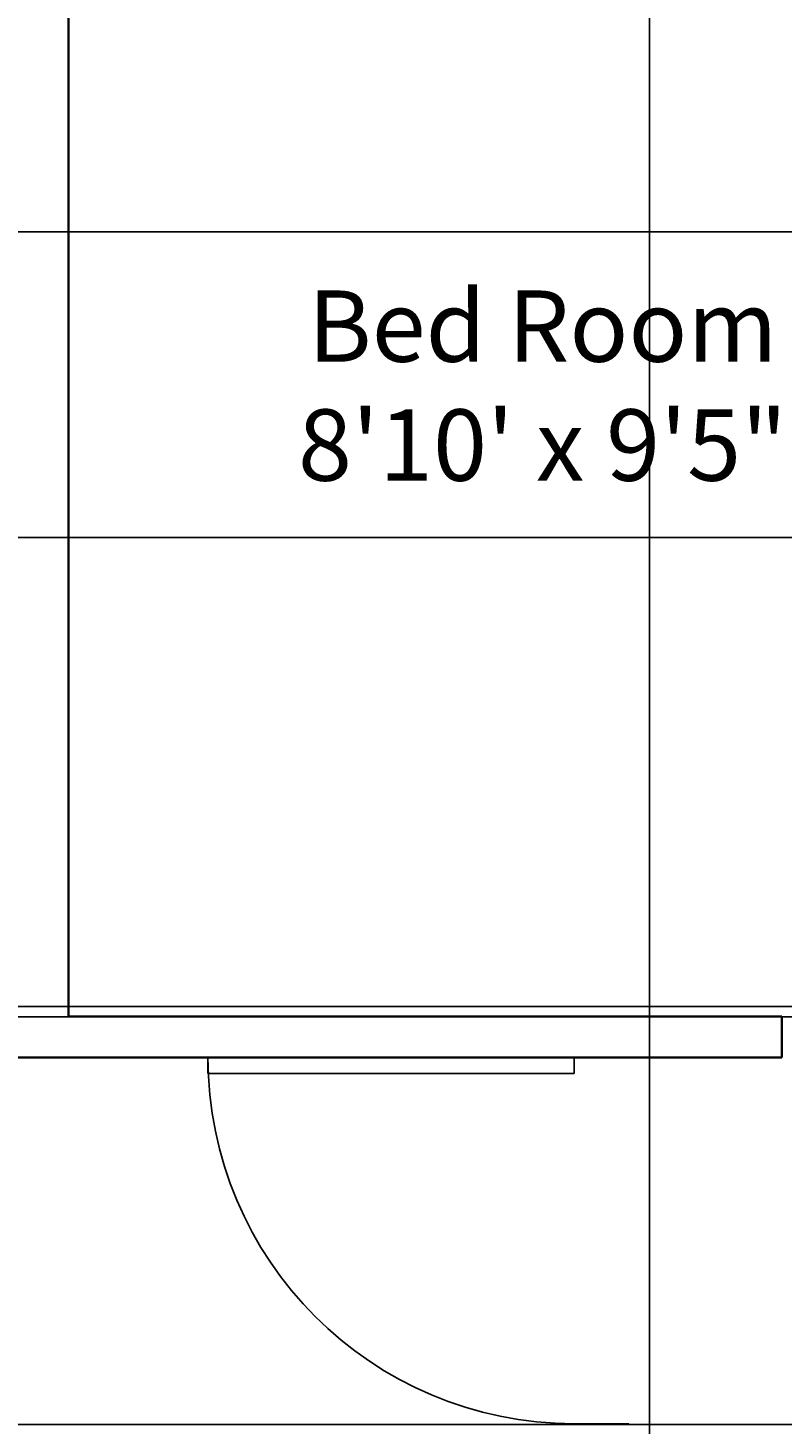
# Model space of a CAD drawing. Units: feet. Extents: x 105 to 1094, y -88 to 588.
# Tile 25 of 59: x 234 to 308, y 354 to 491. Entities that reach past the tile are written whole.
import ezdxf

# ---------------------------------------------------------------- set-up
doc = ezdxf.new("R2010")
doc.units = ezdxf.units.FT
doc.header["$MEASUREMENT"] = 0
for name, color, linetype, lineweight in [('A-ANNO-DIMS', 2, 'Continuous', 18), ('A-AREA-IDEN', 7, 'Continuous', 18), ('A-DOOR', 3, 'Continuous', 25), ('A-WALL', 7, 'Continuous', 35)]:
    doc.layers.add(name, color=color, linetype=linetype, lineweight=lineweight)
doc.styles.get("Standard").update_dxf_attribs({"font": 'arial.ttf'})
doc.dimstyles.get("Standard").update_dxf_attribs({"dimtxt": 0.18, "dimasz": 0.18, "dimexe": 0.18, "dimexo": 0.0625, "dimgap": 0.09, "dimtad": 0, "dimtih": 1, "dimtoh": 1, "dimdec": 4, "dimzin": 0, "dimdsep": 46, "dimtxsty": 'Standard', "dimcen": 0.09, "dimadec": 0, "dimazin": 0, "dimtfac": 1, "dimtdec": 4, "dimtofl": 0, "dimtmove": 0, "dimatfit": 3, "dimfxl": 1, "dimtolj": 1, "dimtzin": 0, "dimarcsym": 0})

# ---------------------------------------------------------------- blocks, each defined once
blk = doc.blocks.new('*U2')
for p, q in [((0, 0), (0, -6)), ((40, 0), (40, -6))]:
    blk.add_line(p, q)
blk.add_lwpolyline([(0, 0), (0, 40), (1.75, 40), (1.75, 0)], close=True)
blk.add_arc((0, 0), 40, 0, 90)
blk = doc.blocks.new('*D21')
at = {"layer": 'A-ANNO-DIMS', "color": 0, "lineweight": -2, "transparency": 16777216}
for p, q in [((849.63, 543.08), (105.46, 543.08)), ((105.64, 542.9), (105.64, 250.26)), ((105.64, -42.74), (105.64, 249.9)), ((849.63, -42.92), (105.46, -42.92))]:
    blk.add_line(p, q, dxfattribs=at)
at = {"layer": 'A-ANNO-DIMS', "color": 0, "transparency": 16777216}
for points in [[(105.61, 542.9), (105.67, 542.9), (105.64, 543.08)], [(105.61, -42.74), (105.67, -42.74), (105.64, -42.92)]]:
    blk.add_solid(points, dxfattribs=at)
at = {"layer": 'Defpoints', "color": 0, "transparency": 16777216}
for p in [(105.64, 543.08), (849.69, 543.08), (849.69, -42.92)]:
    blk.add_point(p, dxfattribs=at)
at = {"layer": 'A-ANNO-DIMS', "color": 0, "transparency": 16777216, "insert": (105.64, 250.08), "char_height": 0.18, "attachment_point": 5}
blk.add_mtext('\\A1;586', dxfattribs=at)
blk = doc.blocks.new('*D32')
at = {"layer": 'A-ANNO-DIMS', "color": 0, "lineweight": -2, "transparency": 16777216}
for p, q in [((646.63, 471.08), (105.46, 471.08)), ((105.64, 470.9), (105.64, 456.26)), ((105.64, 441.26), (105.64, 455.9)), ((646.63, 441.08), (105.46, 441.08))]:
    blk.add_line(p, q, dxfattribs=at)
at = {"layer": 'A-ANNO-DIMS', "color": 0, "transparency": 16777216}
for points in [[(105.61, 470.9), (105.67, 470.9), (105.64, 471.08)], [(105.61, 441.26), (105.67, 441.26), (105.64, 441.08)]]:
    blk.add_solid(points, dxfattribs=at)
at = {"layer": 'Defpoints', "color": 0, "transparency": 16777216}
for p in [(105.64, 471.08), (646.69, 471.08), (646.69, 441.08)]:
    blk.add_point(p, dxfattribs=at)
at = {"layer": 'A-ANNO-DIMS', "color": 0, "transparency": 16777216, "insert": (105.64, 456.08), "char_height": 0.18, "attachment_point": 5}
blk.add_mtext('\\A1;30', dxfattribs=at)
blk = doc.blocks.new('*D33')
at = {"layer": 'A-ANNO-DIMS', "color": 0, "lineweight": -2, "transparency": 16777216}
for p, q in [((646.63, 395.08), (105.46, 395.08)), ((105.64, 394.9), (105.64, 345.26)), ((105.64, 295.26), (105.64, 344.9)), ((646.63, 295.08), (105.46, 295.08))]:
    blk.add_line(p, q, dxfattribs=at)
at = {"layer": 'A-ANNO-DIMS', "color": 0, "transparency": 16777216}
for points in [[(105.61, 394.9), (105.67, 394.9), (105.64, 395.08)], [(105.61, 295.26), (105.67, 295.26), (105.64, 295.08)]]:
    blk.add_solid(points, dxfattribs=at)
at = {"layer": 'Defpoints', "color": 0, "transparency": 16777216}
for p in [(646.69, 395.08), (105.64, 295.08), (646.69, 295.08)]:
    blk.add_point(p, dxfattribs=at)
at = {"layer": 'A-ANNO-DIMS', "color": 0, "transparency": 16777216, "insert": (105.64, 345.08), "char_height": 0.18, "attachment_point": 5}
blk.add_mtext('\\A1;100', dxfattribs=at)
blk = doc.blocks.new('*D38')
at = {"layer": 'A-ANNO-DIMS', "color": 0, "lineweight": -2, "transparency": 16777216}
for p, q in [((150.69, 224.14), (150.69, 588.31)), ((150.87, 588.13), (222.41, 588.13)), ((294.51, 588.13), (222.97, 588.13)), ((294.69, 224.14), (294.69, 588.31))]:
    blk.add_line(p, q, dxfattribs=at)
at = {"layer": 'A-ANNO-DIMS', "color": 0, "transparency": 16777216}
for points in [[(150.87, 588.16), (150.87, 588.1), (150.69, 588.13)], [(294.51, 588.16), (294.51, 588.1), (294.69, 588.13)]]:
    blk.add_solid(points, dxfattribs=at)
at = {"layer": 'Defpoints', "color": 0, "transparency": 16777216}
for p in [(294.69, 588.13), (150.69, 224.08), (294.69, 224.08)]:
    blk.add_point(p, dxfattribs=at)
at = {"layer": 'A-ANNO-DIMS', "color": 0, "transparency": 16777216, "insert": (222.69, 588.13), "char_height": 0.18, "attachment_point": 5}
blk.add_mtext('\\A1;144', dxfattribs=at)
blk = doc.blocks.new('*D39')
at = {"layer": 'A-ANNO-DIMS', "color": 0, "lineweight": -2, "transparency": 16777216}
for p, q in [((294.69, 204.14), (294.69, 588.31)), ((294.87, 588.13), (332.47, 588.13)), ((370.51, 588.13), (332.91, 588.13)), ((370.69, 204.14), (370.69, 588.31))]:
    blk.add_line(p, q, dxfattribs=at)
at = {"layer": 'A-ANNO-DIMS', "color": 0, "transparency": 16777216}
for points in [[(294.87, 588.16), (294.87, 588.1), (294.69, 588.13)], [(370.51, 588.16), (370.51, 588.1), (370.69, 588.13)]]:
    blk.add_solid(points, dxfattribs=at)
at = {"layer": 'Defpoints', "color": 0, "transparency": 16777216}
for p in [(370.69, 588.13), (294.69, 204.08), (370.69, 204.08)]:
    blk.add_point(p, dxfattribs=at)
at = {"layer": 'A-ANNO-DIMS', "color": 0, "transparency": 16777216, "insert": (332.69, 588.13), "char_height": 0.18, "attachment_point": 5}
blk.add_mtext('\\A1;76', dxfattribs=at)
blk = doc.blocks.new('*D51')
at = {"layer": 'A-ANNO-DIMS', "color": 0, "lineweight": -2, "transparency": 16777216}
for p, q in [((432.63, 394.08), (105.46, 394.08)), ((105.64, 393.9), (105.64, 374.26)), ((105.64, 354.26), (105.64, 373.9)), ((426.63, 354.08), (105.46, 354.08))]:
    blk.add_line(p, q, dxfattribs=at)
at = {"layer": 'A-ANNO-DIMS', "color": 0, "transparency": 16777216}
for points in [[(105.61, 393.9), (105.67, 393.9), (105.64, 394.08)], [(105.61, 354.26), (105.67, 354.26), (105.64, 354.08)]]:
    blk.add_solid(points, dxfattribs=at)
at = {"layer": 'Defpoints', "color": 0, "transparency": 16777216}
for p in [(432.69, 394.08), (105.64, 354.08), (426.69, 354.08)]:
    blk.add_point(p, dxfattribs=at)
at = {"layer": 'A-ANNO-DIMS', "color": 0, "transparency": 16777216, "insert": (105.64, 374.08), "char_height": 0.18, "attachment_point": 5}
blk.add_mtext('\\A1;40', dxfattribs=at)

msp = doc.modelspace()

# ---------------------------------------------------------------- linework, layer by layer
at = {"layer": 'A-WALL'}
for p, q in [((237.6883, 507.0812), (237.6883, 394.0812)), ((307.6883, 394.0812), (237.6883, 394.0812)), ((307.6883, 394.0812), (307.6883, 390.0812)), ((307.6883, 390.0812), (156.6883, 390.0812))]:
    msp.add_line(p, q, dxfattribs=at)

# ---------------------------------------------------------------- block references
at = {"layer": 'A-DOOR', "xscale": -0.8984622266767051, "yscale": 0.8984622266767051, "zscale": 0.8984622266767051, "rotation": 90}
msp.add_blockref('*U2', (287.2975, 390.0812), dxfattribs=at)

# ---------------------------------------------------------------- texts
at = {"layer": 'A-AREA-IDEN', "insert": (333.3837, 465.329), "char_height": 7, "attachment_point": 3}
msp.add_mtext_dynamic_manual_height_columns('\\pxqc;Bed Room \\P8\'10\' x 9\'5"', width=98.34246, gutter_width=1, heights=[0], dxfattribs=at)

# ---------------------------------------------------------------- dimensions: what is measured, and where the dimension line sits
at = {"layer": 'A-ANNO-DIMS'}
for base, p1, p2, picture, middle in [((294.6883, 588.1312), (150.6883, 224.0812), (294.6883, 224.0812), '*D38', (222.6883, 588.1312)), ((370.6883, 588.1312), (294.6883, 204.0812), (370.6883, 204.0812), '*D39', (332.6883, 588.1312))]:
    dim = msp.add_linear_dim(base=base, p1=p1, p2=p2, dimstyle='Standard', override={"dimdec": 0, "dimlfac": 1, "dimrnd": 0, "dimzin": 0, "dimdsep": 46, "dimlunit": 2}, dxfattribs=at)
    dim.commit()
    dim.dimension.update_dxf_attribs({"geometry": picture, "text_midpoint": middle})
for base, p1, p2, picture, middle in [((105.6383, 543.0812), (849.6883, -42.9188), (849.6883, 543.0812), '*D21', (105.6383, 250.0812)), ((105.6383, 471.0812), (646.6883, 441.0812), (646.6883, 471.0812), '*D32', (105.6383, 456.0812)), ((105.6383, 295.0812), (646.6883, 395.0812), (646.6883, 295.0812), '*D33', (105.6383, 345.0812)), ((105.6383, 354.0812), (432.6883, 394.0812), (426.6883, 354.0812), '*D51', (105.6383, 374.0812))]:
    dim = msp.add_linear_dim(base=base, p1=p1, p2=p2, angle=90, dimstyle='Standard', override={"dimdec": 0, "dimlfac": 1, "dimrnd": 0, "dimzin": 0, "dimdsep": 46, "dimlunit": 2}, dxfattribs=at)
    dim.commit()
    dim.dimension.update_dxf_attribs({"geometry": picture, "text_midpoint": middle})

doc.saveas('drawing.dxf')
